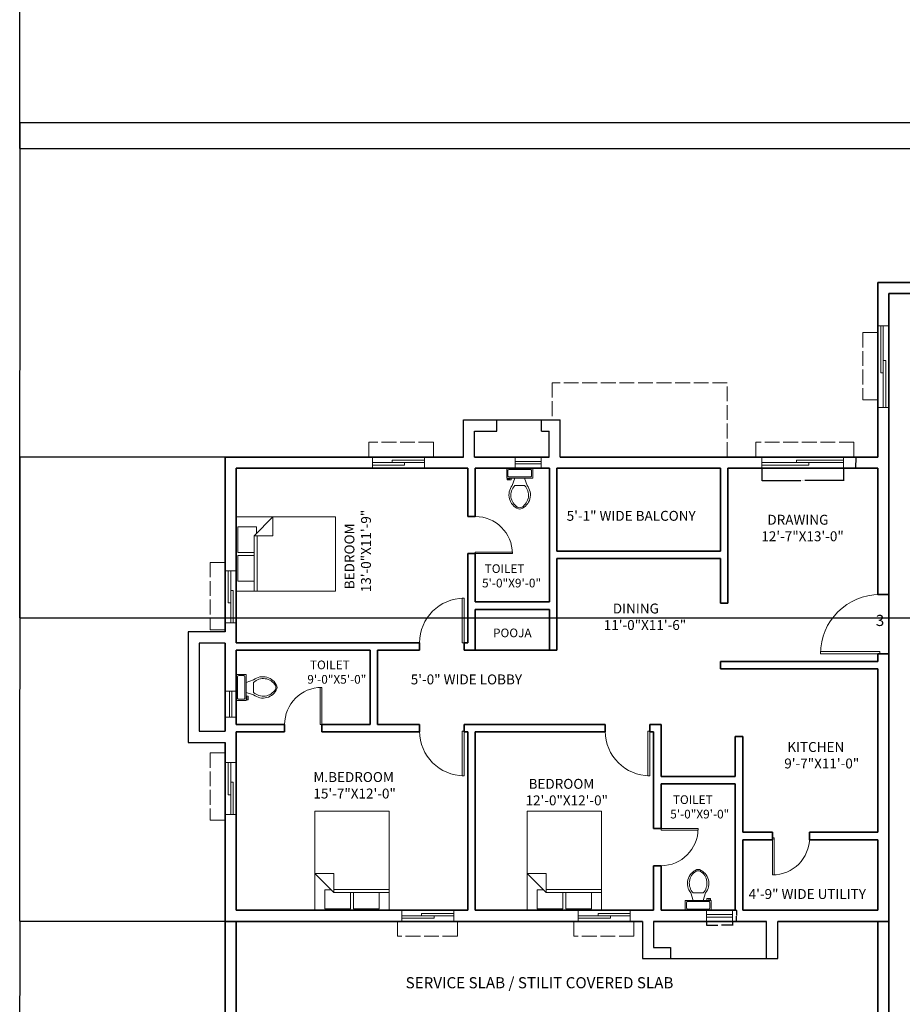
# Model space of a CAD drawing. Units: inches. Extents: x -69 to 2453, y 4803 to 7122.
# Tile 2 of 9: x -69 to 643, y 5448 to 6243. Entities that reach past the tile are written whole.
import ezdxf

# ---------------------------------------------------------------- set-up
doc = ezdxf.new("R2010")
doc.units = ezdxf.units.IN
doc.linetypes.add('ACAD_ISO02W100', pattern=[15, 12, -3])
for name, color, linetype, lineweight in [('A-ANNO-DIMS', 2, 'Continuous', 18), ('A-ANNO-IDEN', 2, 'Continuous', 18), ('A-AREA-IDEN', 7, 'Continuous', 18), ('A-DOOR', 3, 'Continuous', 18), ('A-FLOR-FIXT', 9, 'Continuous', 18), ('A-FLOR-OVHD', 8, 'ACAD_ISO02W100', 13), ('A-FURN', 8, 'Continuous', 18), ('A-GLAZ', 244, 'Continuous', 18), ('A-WALL', 7, 'Continuous', 35), ('A-WALL-SRVC', 7, 'Continuous', 30)]:
    doc.layers.add(name, color=color, linetype=linetype, lineweight=lineweight)
doc.styles.get("Standard").update_dxf_attribs({"font": 'arial.ttf'})
doc.dimstyles.get("Standard").update_dxf_attribs({"dimtxt": 0.18, "dimasz": 0.18, "dimexe": 0.18, "dimexo": 0.0625, "dimgap": 0.09, "dimtad": 0, "dimtih": 1, "dimtoh": 1, "dimdec": 4, "dimzin": 0, "dimdsep": 46, "dimtxsty": 'Standard', "dimcen": 0.09, "dimadec": 0, "dimazin": 0, "dimtfac": 1, "dimtdec": 4, "dimtofl": 0, "dimtmove": 0, "dimatfit": 3, "dimfxl": 1, "dimtolj": 1, "dimtzin": 0, "dimarcsym": 0})

# ---------------------------------------------------------------- blocks, each defined once
blk = doc.blocks.new('*U2')
for p, q in [((-40, 0), (-40, 6)), ((0, 0), (0, 6))]:
    blk.add_line(p, q)
blk.add_lwpolyline([(0, 0), (0, -40), (-1.75, -40), (-1.75, 0)], close=True)
blk.add_arc((0, 0), 40, 180, 270)
blk = doc.blocks.new('*U4')
for p, q in [((0, 0), (0, -6)), ((-40, 0), (-40, -6))]:
    blk.add_line(p, q)
blk.add_lwpolyline([(0, 0), (0, 40), (-1.75, 40), (-1.75, 0)], close=True)
blk.add_arc((0, 0), 40, 90, 180)
blk = doc.blocks.new('*U5')
for p, q in [((0, 0), (0, -6)), ((40, 0), (40, -6))]:
    blk.add_line(p, q)
blk.add_lwpolyline([(0, 0), (0, 40), (1.75, 40), (1.75, 0)], close=True)
blk.add_arc((0, 0), 40, 0, 90)
blk = doc.blocks.new('*U3')
for p, q in [((0, 0), (0, 6)), ((40, 0), (40, 6))]:
    blk.add_line(p, q)
blk.add_lwpolyline([(0, 0), (0, -40), (1.75, -40), (1.75, 0)], close=True)
blk.add_arc((0, 0), 40, 270, 360)
blk = doc.blocks.new('*U6')
for p, q in [((-40, 0), (-40, 6)), ((0, 0), (0, 6))]:
    blk.add_line(p, q)
blk.add_lwpolyline([(0, 0), (0, -40), (-1.75, -40), (-1.75, 0)], close=True)
blk.add_arc((0, 0), 40, 180, 270)
blk = doc.blocks.new('Bed - Queen')
for p, q in [((0, -80.00003), (0, 0)), ((0, 0), (59.99999, 0)), ((59.99999, 0), (59.99999, -80.00003)), ((7.99999, -1.2), (28.79998, -1.2)), ((7.99999, -14.4), (7.99999, -1.2)), ((28.79998, -1.2), (28.79998, -14.4)), ((31.19999, -1.2), (51.99999, -1.2)), ((31.19999, -14.4), (31.19999, -1.2)), ((51.99999, -1.2), (51.99999, -16.4)), ((0, -14.4), (44.8, -14.4)), ((59.99999, -29.6), (44.8, -14.4)), ((44.8, -14.4), (44.8, -29.6)), ((44.8, -16.8), (0, -16.8)), ((51.99999, -16.4), (46.79936, -16.4)), ((44.8, -29.6), (59.99999, -29.6)), ((59.99999, -80.00003), (0, -80.00003))]:
    blk.add_line(p, q)
blk = doc.blocks.new('*U33')
for p, q in [((9.5, -6), (9.5, -2)), ((-10, -8.5), (-8, -8.5)), ((-10, -9.5), (-10, -8.5)), ((-7, -9.5), (-10, -9.5)), ((-8, -8.5), (-8, -8)), ((-7, -8), (-7, -9.5)), ((-4, -8), (-6, -14)), ((4, -14), (-4, -14)), ((4, -8), (6, -14))]:
    blk.add_line(p, q)
blk.add_lwpolyline([(10.5, -8), (10.5, 0), (-10.5, 0), (-10.5, -8)], close=True)
for points in [[(-9.5, -2), (-9.5, -6)], [(8.5, -1), (-8.5, -1)], [(-8.5, -7), (8.5, -7)]]:
    blk.add_lwpolyline(points)
for centre, radius, start, end in [((-8.62, -1.88), 0.884, 81.8699, 188.1301), ((-8.62, -6.12), 0.884, 171.8699, 278.1301), ((8.62, -1.88), 0.884, 351.8699, 98.1301), ((8.62, -6.12), 0.884, 261.8699, 8.1301), ((3.52, -21.58), 12.17, 141.46911, 247.97143), ((4.2, -21.82), 11.33, 136.36773, 238.94682), ((-3.52, -21.58), 12.17, 292.02843, 38.53071), ((-4.2, -21.82), 11.33, 301.05301, 43.63209), ((0, -27.88), 4, 245.73182, 294.26817), ((0, -29), 4, 254.86053, 285.13947)]:
    blk.add_arc(centre, radius, start, end)
blk = doc.blocks.new('WINDOW-VENT-21IN')
for p, q in [((0, 5.5), (21, 5.5)), ((0, 3.5), (21, 3.5))]:
    blk.add_line(p, q)
blk.add_lwpolyline([(0, 9), (21, 9), (21, 0), (0, 0)], close=True)
blk = doc.blocks.new('WINDOW-SLIDING-42IN')
for p, q in [((2.5, 42), (2.5, 16)), ((4.5, 42), (4.5, 0)), ((4.5, 26), (6.5, 26)), ((6.5, 26), (6.5, 0)), ((4.5, 16), (2.5, 16))]:
    blk.add_line(p, q)
blk.add_lwpolyline([(0, 42), (9, 42), (9, 0), (0, 0)], close=True)
blk = doc.blocks.new('WINDOW-SLIDING-66IN')
for p, q in [((66, 4.5), (0, 4.5)), ((38, 2.5), (0, 2.5)), ((66, 6.5), (28, 6.5)), ((28, 4.5), (28, 6.5)), ((38, 4.5), (38, 2.5))]:
    blk.add_line(p, q)
blk.add_lwpolyline([(66, 9), (66, 0), (0, 0), (0, 9)], close=True)
blk = doc.blocks.new('SUNSHADE-54IN')
for p, q in [((12, 54.34), (0, 54.34)), ((0, 54.34), (0, 0)), ((0, 0), (12, 0))]:
    blk.add_line(p, q)
blk = doc.blocks.new('SUNSHADE-48IN')
for p, q in [((0, 0), (0, 12)), ((48.4, 12), (48.4, 0)), ((48.4, 0), (0, 0))]:
    blk.add_line(p, q)
blk = doc.blocks.new('SERVICE-BAY-78IN')
for p, q in [((0, 30), (78.14, 30)), ((0, 0), (0, 30)), ((27.07, 21), (27.07, 30)), ((63.07, 21), (63.07, 30)), ((78.14, 0), (78.14, 30)), ((9, 0), (9, 21)), ((9, 21), (27.07, 21)), ((63.07, 21), (69.14, 21)), ((69.14, 0), (69.14, 21))]:
    blk.add_line(p, q)
blk = doc.blocks.new('*D53')
at = {"layer": 'A-ANNO-DIMS', "color": 0, "lineweight": -2, "transparency": 16777216}
for p, q in [((485.32, 5514.65), (485.32, 5511.39)), ((485.5, 5511.57), (494.33, 5511.57)), ((506.14, 5511.57), (497.3, 5511.57)), ((506.32, 5514.65), (506.32, 5511.39))]:
    blk.add_line(p, q, dxfattribs=at)
at = {"layer": 'A-ANNO-DIMS', "color": 0, "transparency": 16777216}
for points in [[(485.5, 5511.6), (485.5, 5511.54), (485.32, 5511.57)], [(506.14, 5511.6), (506.14, 5511.54), (506.32, 5511.57)]]:
    blk.add_solid(points, dxfattribs=at)
at = {"layer": 'Defpoints', "color": 0, "transparency": 16777216}
for p in [(485.32, 5514.72), (506.32, 5514.72), (506.32, 5511.57)]:
    blk.add_point(p, dxfattribs=at)
at = {"layer": 'A-ANNO-DIMS', "color": 0, "transparency": 16777216, "insert": (495.82, 5511.57), "char_height": 0.18, "attachment_point": 5}
blk.add_mtext('\\A1;VENT WINDOW 21 TYP.', dxfattribs=at)
blk = doc.blocks.new('*D54')
at = {"layer": 'A-ANNO-DIMS', "color": 0, "lineweight": -2, "transparency": 16777216}
for p, q in [((506.38, 5523.72), (509.65, 5523.72)), ((509.47, 5523.54), (509.47, 5519.4)), ((509.47, 5514.9), (509.47, 5519.03)), ((506.38, 5514.72), (509.65, 5514.72))]:
    blk.add_line(p, q, dxfattribs=at)
at = {"layer": 'A-ANNO-DIMS', "color": 0, "transparency": 16777216}
for points in [[(509.44, 5523.54), (509.5, 5523.54), (509.47, 5523.72)], [(509.44, 5514.9), (509.5, 5514.9), (509.47, 5514.72)]]:
    blk.add_solid(points, dxfattribs=at)
at = {"layer": 'Defpoints', "color": 0, "transparency": 16777216}
for p in [(506.32, 5523.72), (509.47, 5523.72), (506.32, 5514.72)]:
    blk.add_point(p, dxfattribs=at)
at = {"layer": 'A-ANNO-DIMS', "color": 0, "transparency": 16777216, "insert": (509.47, 5519.22), "char_height": 0.18, "attachment_point": 5}
blk.add_mtext('\\A1;9 TYP.', dxfattribs=at)
blk = doc.blocks.new('*D57')
at = {"layer": 'A-ANNO-DIMS', "color": 0, "lineweight": -2, "transparency": 16777216}
for p, q in [((530.01, 5880.65), (530.01, 5870.64)), ((596.01, 5880.65), (596.01, 5870.64)), ((530.19, 5870.82), (561.36, 5870.82)), ((595.83, 5870.82), (564.66, 5870.82))]:
    blk.add_line(p, q, dxfattribs=at)
at = {"layer": 'A-ANNO-DIMS', "color": 0, "transparency": 16777216}
for points in [[(530.19, 5870.85), (530.19, 5870.79), (530.01, 5870.82)], [(595.83, 5870.85), (595.83, 5870.79), (596.01, 5870.82)]]:
    blk.add_solid(points, dxfattribs=at)
at = {"layer": 'Defpoints', "color": 0, "transparency": 16777216}
for p in [(530.01, 5880.72), (596.01, 5880.72), (596.01, 5870.82)]:
    blk.add_point(p, dxfattribs=at)
at = {"layer": 'A-ANNO-DIMS', "color": 0, "transparency": 16777216, "insert": (563.01, 5870.82), "char_height": 0.18, "attachment_point": 5}
blk.add_mtext('\\A1;SLIDING WINDOW 66 TYP.', dxfattribs=at)
blk = doc.blocks.new('*D58')
at = {"layer": 'A-ANNO-DIMS', "color": 0, "lineweight": -2, "transparency": 16777216}
for p, q in [((596.07, 5889.72), (606.09, 5889.72)), ((605.91, 5889.54), (605.91, 5885.4)), ((605.91, 5880.9), (605.91, 5885.03)), ((596.07, 5880.72), (606.09, 5880.72))]:
    blk.add_line(p, q, dxfattribs=at)
at = {"layer": 'A-ANNO-DIMS', "color": 0, "transparency": 16777216}
for points in [[(605.88, 5889.54), (605.94, 5889.54), (605.91, 5889.72)], [(605.88, 5880.9), (605.94, 5880.9), (605.91, 5880.72)]]:
    blk.add_solid(points, dxfattribs=at)
at = {"layer": 'Defpoints', "color": 0, "transparency": 16777216}
for p in [(596.01, 5889.72), (605.91, 5889.72), (596.01, 5880.72)]:
    blk.add_point(p, dxfattribs=at)
at = {"layer": 'A-ANNO-DIMS', "color": 0, "transparency": 16777216, "insert": (605.91, 5885.22), "char_height": 0.18, "attachment_point": 5}
blk.add_mtext('\\A1;9 TYP.', dxfattribs=at)
blk = doc.blocks.new('*D98')
at = {"layer": 'A-ANNO-DIMS', "color": 0, "lineweight": -2, "transparency": 16777216}
for p, q in [((96.45, 5514.72), (-69.42, 5514.72)), ((-69.24, 5514.54), (-69.24, 5454.9)), ((-69.24, 5394.9), (-69.24, 5454.53)), ((96.45, 5394.72), (-69.42, 5394.72))]:
    blk.add_line(p, q, dxfattribs=at)
at = {"layer": 'A-ANNO-DIMS', "color": 0, "transparency": 16777216}
for points in [[(-69.27, 5514.54), (-69.21, 5514.54), (-69.24, 5514.72)], [(-69.27, 5394.9), (-69.21, 5394.9), (-69.24, 5394.72)]]:
    blk.add_solid(points, dxfattribs=at)
at = {"layer": 'Defpoints', "color": 0, "transparency": 16777216}
for p in [(-69.24, 5514.72), (96.51, 5514.72), (96.51, 5394.72)]:
    blk.add_point(p, dxfattribs=at)
at = {"layer": 'A-ANNO-DIMS', "color": 0, "transparency": 16777216, "insert": (-69.24, 5454.72), "char_height": 0.18, "attachment_point": 5}
blk.add_mtext('\\A1;120', dxfattribs=at)
blk = doc.blocks.new('*D99')
at = {"layer": 'A-ANNO-DIMS', "color": 0, "lineweight": -2, "transparency": 16777216}
for p, q in [((96.45, 5889.72), (-69.42, 5889.72)), ((-69.24, 5889.54), (-69.24, 5702.4)), ((-69.24, 5514.9), (-69.24, 5702.03)), ((96.45, 5514.72), (-69.42, 5514.72))]:
    blk.add_line(p, q, dxfattribs=at)
at = {"layer": 'A-ANNO-DIMS', "color": 0, "transparency": 16777216}
for points in [[(-69.27, 5889.54), (-69.21, 5889.54), (-69.24, 5889.72)], [(-69.27, 5514.9), (-69.21, 5514.9), (-69.24, 5514.72)]]:
    blk.add_solid(points, dxfattribs=at)
at = {"layer": 'Defpoints', "color": 0, "transparency": 16777216}
for p in [(-69.24, 5889.72), (96.51, 5889.72), (96.51, 5514.72)]:
    blk.add_point(p, dxfattribs=at)
at = {"layer": 'A-ANNO-DIMS', "color": 0, "transparency": 16777216, "insert": (-69.24, 5702.22), "char_height": 0.18, "attachment_point": 5}
blk.add_mtext('\\A1;375', dxfattribs=at)
blk = doc.blocks.new('*D101')
at = {"layer": 'A-ANNO-DIMS', "color": 0, "lineweight": -2, "transparency": 16777216}
for p, q in [((752.45, 6159.72), (-69.42, 6159.72)), ((-69.24, 6159.54), (-69.24, 5959.9)), ((-69.24, 5759.9), (-69.24, 5959.53)), ((761.45, 5759.72), (-69.42, 5759.72))]:
    blk.add_line(p, q, dxfattribs=at)
at = {"layer": 'A-ANNO-DIMS', "color": 0, "transparency": 16777216}
for points in [[(-69.27, 6159.54), (-69.21, 6159.54), (-69.24, 6159.72)], [(-69.27, 5759.9), (-69.21, 5759.9), (-69.24, 5759.72)]]:
    blk.add_solid(points, dxfattribs=at)
at = {"layer": 'Defpoints', "color": 0, "transparency": 16777216}
for p in [(-69.24, 6159.72), (752.51, 6159.72), (761.51, 5759.72)]:
    blk.add_point(p, dxfattribs=at)
at = {"layer": 'A-ANNO-DIMS', "color": 0, "transparency": 16777216, "insert": (-69.24, 5959.72), "char_height": 0.18, "attachment_point": 5}
blk.add_mtext('\\A1;400', dxfattribs=at)
blk = doc.blocks.new('*D103')
at = {"layer": 'A-ANNO-DIMS', "color": 0, "lineweight": -2, "transparency": 16777216}
for p, q in [((1241.45, 6552.72), (-69.42, 6552.72)), ((-69.24, 6552.54), (-69.24, 6345.9)), ((-69.24, 6138.9), (-69.24, 6345.53)), ((1241.45, 6138.72), (-69.42, 6138.72))]:
    blk.add_line(p, q, dxfattribs=at)
at = {"layer": 'A-ANNO-DIMS', "color": 0, "transparency": 16777216}
for points in [[(-69.27, 6552.54), (-69.21, 6552.54), (-69.24, 6552.72)], [(-69.27, 6138.9), (-69.21, 6138.9), (-69.24, 6138.72)]]:
    blk.add_solid(points, dxfattribs=at)
at = {"layer": 'Defpoints', "color": 0, "transparency": 16777216}
for p in [(-69.24, 6552.72), (1241.51, 6552.72), (1241.51, 6138.72)]:
    blk.add_point(p, dxfattribs=at)
at = {"layer": 'A-ANNO-DIMS', "color": 0, "transparency": 16777216, "insert": (-69.24, 6345.72), "char_height": 0.18, "attachment_point": 5}
blk.add_mtext('\\A1;414', dxfattribs=at)

msp = doc.modelspace()

# ---------------------------------------------------------------- linework, layer by layer
at = {"layer": 'A-FLOR-OVHD'}
for p, q in [((501.97, 5949.72), (360.55, 5949.72)), ((360.55, 5949.72), (360.55, 5919.72)), ((501.97, 5889.72), (501.97, 5949.72)), ((264.78, 5901.72), (212.46, 5901.72)), ((212.46, 5901.72), (212.46, 5889.72)), ((264.78, 5889.72), (264.78, 5901.72)), ((604.28, 5901.72), (525.06, 5901.72)), ((525.06, 5901.72), (525.06, 5889.72)), ((604.28, 5889.72), (604.28, 5901.72)), ((96.51, 5650.87), (84.51, 5650.87)), ((84.51, 5650.87), (84.51, 5596.5)), ((84.51, 5596.5), (96.51, 5596.5))]:
    msp.add_line(p, q, dxfattribs=at)
at = {"layer": 'A-WALL'}
for p, q in [((623.51, 6030.72), (623.51, 5889.72)), ((623.51, 6030.72), (752.51, 6030.72)), ((632.51, 6021.72), (752.51, 6021.72)), ((632.51, 6021.72), (632.51, 5328.72)), ((96.51, 5889.72), (96.51, 5748.47)), ((96.51, 5889.72), (288.94, 5889.72)), ((297.94, 5889.72), (358.08, 5889.72)), ((367.08, 5889.72), (623.51, 5889.72)), ((105.51, 5880.72), (292.51, 5880.72)), ((105.51, 5880.72), (105.51, 5739.72)), ((292.51, 5880.72), (292.51, 5841.72)), ((298.51, 5880.72), (298.51, 5841.72)), ((298.51, 5880.72), (358.51, 5880.72)), ((358.51, 5880.72), (358.51, 5772.72)), ((364.51, 5880.72), (364.51, 5813.72)), ((364.51, 5880.72), (496.51, 5880.72)), ((496.51, 5880.72), (496.51, 5813.72)), ((502.51, 5880.72), (502.51, 5771.72)), ((502.51, 5880.72), (623.51, 5880.72)), ((623.51, 5880.72), (623.51, 5778.72)), ((298.51, 5841.72), (292.51, 5841.72)), ((364.51, 5813.72), (496.51, 5813.72)), ((298.51, 5811.72), (292.51, 5811.72)), ((292.51, 5811.72), (292.51, 5739.72)), ((298.51, 5811.72), (298.51, 5772.72)), ((364.51, 5807.72), (496.51, 5807.72)), ((364.51, 5807.72), (364.51, 5733.72)), ((496.51, 5807.72), (496.51, 5771.72)), ((298.51, 5772.72), (358.51, 5772.72)), ((623.51, 5778.72), (632.51, 5778.72)), ((298.51, 5766.72), (358.51, 5766.72)), ((298.51, 5766.72), (298.51, 5733.72)), ((358.51, 5766.72), (358.51, 5733.72)), ((496.51, 5771.72), (502.51, 5771.72)), ((96.51, 5739.47), (96.51, 5668.27)), ((105.51, 5739.72), (253.51, 5739.72)), ((105.51, 5733.72), (213.51, 5733.72)), ((105.51, 5733.72), (105.51, 5673.72)), ((213.51, 5733.72), (213.51, 5673.72)), ((219.51, 5733.72), (219.51, 5673.72)), ((219.51, 5733.72), (253.51, 5733.72)), ((253.51, 5739.72), (253.51, 5733.72)), ((289.51, 5739.72), (289.51, 5733.72)), ((289.51, 5739.72), (292.51, 5739.72)), ((289.51, 5733.72), (364.51, 5733.72)), ((623.51, 5730.72), (632.51, 5730.72)), ((623.51, 5730.72), (623.51, 5724.72)), ((496.51, 5724.72), (623.51, 5724.72)), ((496.51, 5724.72), (496.51, 5718.72)), ((496.51, 5718.72), (623.51, 5718.72)), ((623.51, 5718.72), (623.51, 5586.72)), ((105.51, 5673.72), (144.51, 5673.72)), ((144.51, 5673.72), (144.51, 5667.72)), ((174.51, 5673.72), (174.51, 5667.72)), ((174.51, 5673.72), (213.51, 5673.72)), ((219.51, 5673.72), (253.51, 5673.72)), ((253.51, 5667.72), (253.51, 5673.72)), ((289.51, 5667.72), (289.51, 5673.72)), ((289.51, 5673.72), (403.51, 5673.72)), ((403.51, 5667.72), (403.51, 5673.72)), ((439.51, 5667.72), (439.51, 5673.72)), ((439.51, 5673.72), (448.51, 5673.72)), ((448.51, 5673.72), (448.51, 5631.72)), ((105.51, 5667.72), (144.51, 5667.72)), ((105.51, 5667.72), (105.51, 5523.72)), ((174.51, 5667.72), (253.51, 5667.72)), ((289.51, 5667.72), (292.51, 5667.72)), ((292.51, 5667.72), (292.51, 5523.72)), ((298.51, 5667.72), (403.51, 5667.72)), ((298.51, 5667.72), (298.51, 5523.72)), ((439.51, 5667.72), (442.51, 5667.72)), ((442.51, 5667.72), (442.51, 5589.72)), ((508.51, 5663.99), (508.51, 5631.72)), ((514.51, 5663.99), (508.51, 5663.99)), ((514.51, 5663.99), (514.51, 5586.72)), ((96.51, 5659.27), (96.51, 5020.72)), ((448.51, 5631.72), (508.51, 5631.72)), ((448.51, 5625.72), (508.51, 5625.72)), ((448.51, 5625.72), (448.51, 5589.72)), ((508.51, 5625.72), (508.51, 5523.72)), ((448.51, 5589.72), (442.51, 5589.72)), ((514.51, 5586.72), (538.51, 5586.72)), ((538.51, 5580.72), (538.51, 5586.72)), ((568.51, 5580.72), (568.51, 5586.72)), ((568.51, 5586.72), (623.51, 5586.72)), ((514.51, 5580.72), (538.51, 5580.72)), ((514.51, 5580.72), (514.51, 5523.72)), ((568.51, 5580.72), (623.51, 5580.72)), ((623.51, 5580.72), (623.51, 5523.72)), ((448.51, 5559.72), (442.51, 5559.72)), ((442.51, 5559.72), (442.51, 5523.72)), ((448.51, 5559.72), (448.51, 5523.72)), ((105.51, 5523.72), (292.51, 5523.72)), ((298.51, 5523.72), (442.51, 5523.72)), ((448.51, 5523.72), (508.51, 5523.72)), ((514.51, 5523.72), (623.51, 5523.72)), ((96.51, 5514.72), (433.51, 5514.72)), ((105.51, 5514.72), (105.51, 5394.72)), ((442.51, 5514.72), (533.8, 5514.72)), ((542.8, 5514.72), (632.51, 5514.72)), ((623.51, 5514.72), (623.51, 5394.72))]:
    msp.add_line(p, q, dxfattribs=at)
at = {"layer": 'A-WALL-SRVC'}
for p, q in [((66.51, 5748.47), (66.51, 5659.27)), ((96.51, 5748.47), (66.51, 5748.47)), ((96.51, 5739.47), (75.51, 5739.47)), ((75.51, 5739.47), (75.51, 5668.27)), ((75.51, 5668.27), (96.51, 5668.27)), ((66.51, 5659.27), (96.51, 5659.27)), ((433.51, 5514.72), (433.51, 5484.72)), ((442.51, 5514.72), (442.51, 5493.72)), ((533.8, 5484.72), (533.8, 5514.72)), ((542.8, 5484.72), (542.8, 5514.72)), ((442.51, 5493.72), (456.12, 5493.72)), ((456.12, 5493.72), (456.12, 5484.72)), ((433.51, 5484.72), (542.8, 5484.72))]:
    msp.add_line(p, q, dxfattribs=at)

# ---------------------------------------------------------------- block references
at = {"layer": 'A-DOOR', "rotation": 270.0000000000001}
for name, p, xscale, yscale, zscale in [('*U4', (298.51, 5811.72), 0.75, 0.75, 0.75), ('*U6', (625.31, 5730.72), 1.199999999999977, 1.199999999999977, 1.199999999999977), ('*U5', (448.51, 5589.72), 0.75, 0.75, 0.75)]:
    msp.add_blockref(name, p, dxfattribs=dict(at, xscale=xscale, yscale=yscale, zscale=zscale))
at = {"layer": 'A-DOOR'}
for name, p, xscale, yscale, zscale in [('*U4', (289.51, 5739.72), 0.9, 0.9, 0.9), ('*U4', (174.51, 5673.72), 0.75, 0.75, 0.75), ('*U2', (289.51, 5668.32), 0.9, 0.9, 0.9), ('*U2', (439.51, 5668.32), 0.9, 0.9, 0.9), ('*U3', (538.51, 5582.22), 0.7500000000000029, 0.7500000000000029, 0.7500000000000029)]:
    msp.add_blockref(name, p, dxfattribs=dict(at, xscale=xscale, yscale=yscale, zscale=zscale))
at = {"layer": 'A-FLOR-FIXT'}
msp.add_blockref('*U33', (334.38, 5880.72), dxfattribs=at)
for p, rotation in [((105.51, 5703.72), 89.99999999999999), ((478.51, 5523.72), 180)]:
    msp.add_blockref('*U33', p, dxfattribs=dict(at, rotation=rotation))
at = {"layer": 'A-FLOR-OVHD'}
for name, p in [('SUNSHADE-54IN', (611.51, 5935.97)), ('SUNSHADE-54IN', (84.51, 5750.27)), ('SUNSHADE-48IN', (235.75, 5502.72)), ('SUNSHADE-48IN', (378.2, 5502.72))]:
    msp.add_blockref(name, p, dxfattribs=at)
at = {"layer": 'A-FURN'}
for p, rotation in [((105.51, 5781.42), 89.99999999999999), ((229.01, 5523.72), 180), ((400.51, 5523.72), 180)]:
    msp.add_blockref('Bed - Queen', p, dxfattribs=dict(at, rotation=rotation))
at = {"layer": 'A-GLAZ'}
for name, p, rotation in [('WINDOW-SLIDING-66IN', (632.51, 5929.62), 89.99999999999987), ('WINDOW-SLIDING-42IN', (215.42, 5889.72), 269.9999999999985), ('WINDOW-VENT-21IN', (96.51, 5700.68), 269.9999999999973), ('WINDOW-SLIDING-42IN', (239.21, 5523.72), 269.9999999999962), ('WINDOW-SLIDING-42IN', (381.65, 5523.72), 269.9999999999962)]:
    msp.add_blockref(name, p, dxfattribs=dict(at, rotation=rotation))
for name, p in [('WINDOW-VENT-21IN', (330.81, 5880.72)), ('WINDOW-SLIDING-66IN', (530.01, 5880.72)), ('WINDOW-SLIDING-42IN', (96.51, 5755.92)), ('WINDOW-SLIDING-42IN', (96.51, 5601.05)), ('WINDOW-VENT-21IN', (485.32, 5514.72))]:
    msp.add_blockref(name, p, dxfattribs=at)
at = {"layer": 'A-WALL-SRVC'}
msp.add_blockref('SERVICE-BAY-78IN', (288.94, 5889.72), dxfattribs=at)

# ---------------------------------------------------------------- texts
at = {"layer": 'A-ANNO-IDEN', "insert": (622.01, 5762.27), "char_height": 8, "attachment_point": 1}
msp.add_mtext_dynamic_manual_height_columns('{\\H1.125x;3} ', width=10.4994, gutter_width=12.5, heights=[0], dxfattribs=at)
at = {"layer": 'A-AREA-IDEN', "insert": (192.89, 5780.56), "char_height": 8, "attachment_point": 1, "rotation": 90}
msp.add_mtext_dynamic_manual_height_columns(' BEDROOM\\P13\'-0"X11\'-9"', width=64.9911, gutter_width=12.5, heights=[0], dxfattribs=at)
at = {"layer": 'A-AREA-IDEN', "attachment_point": 1}
for s, width, insert, char_height in [('5\'-1" WIDE BALCONY', 114.3745, (372.32, 5846.25), 8), ('  DRAWING\\P12\'-7"X13\'-0"', 64.9911, (529.55, 5843.09), 8), (' TOILET\\P5\'-0"X9\'-0"', 51.0295, (303.97, 5803.12), 7), ('   DINING\\P11\'-0"X11\'-6"', 63.2359, (402.27, 5771.4), 8), ('POOJA', 33.9191, (312.86, 5751.21), 7), (' TOILET\\P9\'-0"X5\'-0"', 45.2002, (162.85, 5725.37), 7), ('5\'-0" WIDE LOBBY', 96.5666, (246.39, 5714.14), 8), (' KITCHEN\\P9\'-7"X11\'-0"', 58.1282, (548.07, 5659.59), 8), ('M.BEDROOM\\P15\'-7"X12\'-0"', 69.6032, (167.78, 5635.32), 8), (' BEDROOM\\P12\'-0"X12\'-0"', 64.9911, (339.11, 5629.82), 8), (' TOILET\\P5\'-0"X9\'-0"', 45.2514, (455.97, 5616.55), 7), ('4\'-9" WIDE UTILITY', 99.5525, (519.29, 5540.84), 8), ('SERVICE SLAB / STILIT COVERED SLAB', 244.2019, (242.25, 5469.71), 9)]:
    msp.add_mtext_dynamic_manual_height_columns(s, width=width, gutter_width=12.5, heights=[0], dxfattribs=dict(at, insert=insert, char_height=char_height))

# ---------------------------------------------------------------- dimensions: what is measured, and where the dimension line sits
at = {"layer": 'A-ANNO-DIMS'}
for base, p1, p2, picture, middle in [((-69.24, 6552.72), (1241.51, 6138.72), (1241.51, 6552.72), '*D103', (-69.24, 6345.72)), ((-69.24, 6159.72), (761.51, 5759.72), (752.51, 6159.72), '*D101', (-69.24, 5959.72)), ((-69.24, 5889.72), (96.51, 5514.72), (96.51, 5889.72), '*D99', (-69.24, 5702.22)), ((-69.24, 5514.72), (96.51, 5394.72), (96.51, 5514.72), '*D98', (-69.24, 5454.72))]:
    dim = msp.add_linear_dim(base=base, p1=p1, p2=p2, angle=90, dimstyle='Standard', override={"dimdec": 0, "dimlfac": 1, "dimrnd": 0, "dimzin": 0, "dimdsep": 46, "dimlunit": 2}, dxfattribs=at)
    dim.commit()
    dim.dimension.update_dxf_attribs({"geometry": picture, "text_midpoint": middle})
for base, p1, p2, picture, middle in [((605.91, 5889.72), (596.01, 5880.72), (596.01, 5889.72), '*D58', (605.91, 5885.22)), ((509.47, 5523.72), (506.32, 5514.72), (506.32, 5523.72), '*D54', (509.47, 5519.22))]:
    dim = msp.add_linear_dim(base=base, p1=p1, p2=p2, angle=90, text='<> TYP.', dimstyle='Standard', override={"dimdec": 0, "dimlfac": 1, "dimrnd": 0, "dimzin": 0, "dimdsep": 46, "dimlunit": 2}, dxfattribs=at)
    dim.commit()
    dim.dimension.update_dxf_attribs({"geometry": picture, "text_midpoint": middle})
for base, p1, p2, text, picture, middle in [((596.01, 5870.82), (530.01, 5880.72), (596.01, 5880.72), 'SLIDING WINDOW <> TYP.', '*D57', (563.01, 5870.82)), ((506.32, 5511.57), (485.32, 5514.72), (506.32, 5514.72), 'VENT WINDOW <> TYP.', '*D53', (495.82, 5511.57))]:
    dim = msp.add_linear_dim(base=base, p1=p1, p2=p2, text=text, dimstyle='Standard', override={"dimdec": 0, "dimlfac": 1, "dimrnd": 0, "dimzin": 0, "dimdsep": 46, "dimlunit": 2}, dxfattribs=at)
    dim.commit()
    dim.dimension.update_dxf_attribs({"geometry": picture, "text_midpoint": middle})

doc.saveas('drawing.dxf')
